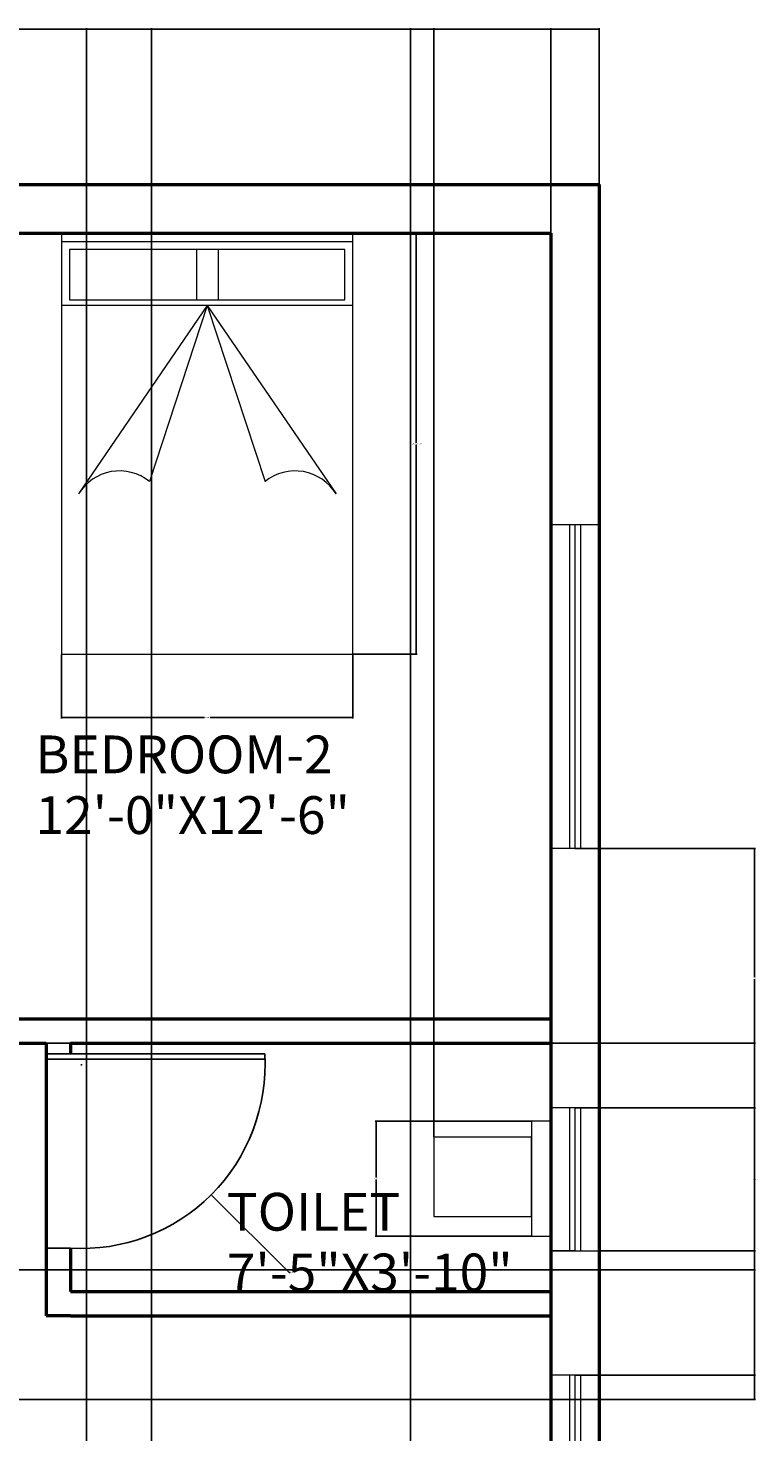
# Model space of a CAD drawing. Units: inches. Extents: x 2750 to 3097, y 1429 to 2028.
# Tile 4 of 4: x 2962 to 3097, y 1768 to 2028. Entities that reach past the tile are written whole.
import ezdxf

# ---------------------------------------------------------------- set-up
doc = ezdxf.new("R2010")
doc.units = ezdxf.units.IN
for name, color, linetype, lineweight in [('A-ANNO-DIMS', 2, 'Continuous', 18), ('A-AREA-IDEN', 7, 'Continuous', 25), ('A-DOOR', 3, 'Continuous', 25), ('A-FLOR-FIXT', 9, 'Continuous', 18), ('A-FURN', 8, 'Continuous', 18), ('A-GLAZ', 4, 'Continuous', 18), ('A-WALL', 7, 'Continuous', 50)]:
    doc.layers.add(name, color=color, linetype=linetype, lineweight=lineweight)
doc.styles.get("Standard").update_dxf_attribs({"font": 'arial.ttf'})
doc.dimstyles.get("Standard").update_dxf_attribs({"dimtxt": 0.18, "dimasz": 0.18, "dimexe": 0.18, "dimexo": 0.0625, "dimgap": 0.09, "dimtad": 0, "dimtih": 1, "dimtoh": 1, "dimdec": 4, "dimzin": 0, "dimdsep": 46, "dimtxsty": 'Standard', "dimcen": 0.09, "dimadec": 0, "dimazin": 0, "dimtfac": 1, "dimtdec": 4, "dimtofl": 0, "dimtmove": 0, "dimatfit": 3, "dimfxl": 1, "dimtolj": 1, "dimtzin": 0, "dimarcsym": 0})

# ---------------------------------------------------------------- blocks, each defined once
blk = doc.blocks.new('BED-DOUBLE-54X78')
for p, q in [((0, 78), (0, 0)), ((54, 78), (0, 78)), ((54, 0), (54, 78)), ((27, 13.39), (3.13, 48.31)), ((27, 13.39), (50.87, 48.31)), ((27, 13.39), (16.28, 45.98)), ((27, 13.39), (37.72, 45.98)), ((0, 13.39), (54, 13.39)), ((24.99, 3.04), (24.99, 12.35)), ((28.99, 3.04), (28.99, 12.35)), ((0, 1.59), (54, 1.59)), ((0, 0), (54, 0))]:
    blk.add_line(p, q)
blk.add_lwpolyline([(1.48, 3.04), (52.5, 3.04), (52.5, 12.35), (1.48, 12.35)], close=True)
for centre, start, end in [((10.73, 52.93), 211.2898, 308.6091), ((43.27, 52.93), 231.3909, 328.7102)]:
    blk.add_arc(centre, 8.89, start, end)
blk = doc.blocks.new('WIN-60IN')
for p, q in [((9, 60), (0, 60)), ((3.5, 60), (3.5, 0)), ((4.5, 60), (4.5, 0)), ((5.5, 60), (5.5, 0)), ((9, 0), (0, 0))]:
    blk.add_line(p, q)
blk = doc.blocks.new('*D9')
at = {"layer": 'A-ANNO-DIMS', "color": 0, "lineweight": -2, "transparency": 16777216}
for p, q in [((3021.93, 1989.59), (3033.75, 1989.59)), ((3033.57, 1989.41), (3033.57, 1950.78)), ((3033.57, 1911.77), (3033.57, 1950.41)), ((3021.93, 1911.59), (3033.75, 1911.59))]:
    blk.add_line(p, q, dxfattribs=at)
at = {"layer": 'A-ANNO-DIMS', "color": 0, "transparency": 16777216}
for points in [[(3033.54, 1989.41), (3033.6, 1989.41), (3033.57, 1989.59)], [(3033.54, 1911.77), (3033.6, 1911.77), (3033.57, 1911.59)]]:
    blk.add_solid(points, dxfattribs=at)
at = {"layer": 'Defpoints', "color": 0, "transparency": 16777216}
for p in [(3021.87, 1989.59), (3021.87, 1911.59), (3033.57, 1911.59)]:
    blk.add_point(p, dxfattribs=at)
at = {"layer": 'A-ANNO-DIMS', "color": 0, "transparency": 16777216, "insert": (3033.57, 1950.59), "char_height": 0.18, "attachment_point": 5}
blk.add_mtext('\\A1;DOUBLE BED 78 TYP.', dxfattribs=at)
blk = doc.blocks.new('*D10')
at = {"layer": 'A-ANNO-DIMS', "color": 0, "lineweight": -2, "transparency": 16777216}
for p, q in [((2967.87, 1911.53), (2967.87, 1899.71)), ((3021.87, 1911.53), (3021.87, 1899.71)), ((2968.05, 1899.89), (2994.34, 1899.89)), ((3021.69, 1899.89), (2995.4, 1899.89))]:
    blk.add_line(p, q, dxfattribs=at)
at = {"layer": 'A-ANNO-DIMS', "color": 0, "transparency": 16777216}
for points in [[(2968.05, 1899.92), (2968.05, 1899.86), (2967.87, 1899.89)], [(3021.69, 1899.92), (3021.69, 1899.86), (3021.87, 1899.89)]]:
    blk.add_solid(points, dxfattribs=at)
at = {"layer": 'Defpoints', "color": 0, "transparency": 16777216}
for p in [(2967.87, 1911.59), (3021.87, 1911.59), (2967.87, 1899.89)]:
    blk.add_point(p, dxfattribs=at)
at = {"layer": 'A-ANNO-DIMS', "color": 0, "transparency": 16777216, "insert": (2994.87, 1899.89), "char_height": 0.18, "attachment_point": 5}
blk.add_mtext('\\A1;54 TYP.', dxfattribs=at)
blk = doc.blocks.new('*D13')
at = {"layer": 'A-ANNO-DIMS', "color": 0, "lineweight": -2, "transparency": 16777216}
for p, q in [((2779.52, 1998.66), (2779.52, 2027.57)), ((2779.7, 2027.39), (2923.23, 2027.39)), ((3067.34, 2027.39), (2923.81, 2027.39)), ((3067.52, 1998.66), (3067.52, 2027.57))]:
    blk.add_line(p, q, dxfattribs=at)
at = {"layer": 'A-ANNO-DIMS', "color": 0, "transparency": 16777216}
for points in [[(2779.7, 2027.42), (2779.7, 2027.36), (2779.52, 2027.39)], [(3067.34, 2027.42), (3067.34, 2027.36), (3067.52, 2027.39)]]:
    blk.add_solid(points, dxfattribs=at)
at = {"layer": 'Defpoints', "color": 0, "transparency": 16777216}
for p in [(3067.52, 2027.39), (2779.52, 1998.59), (3067.52, 1998.59)]:
    blk.add_point(p, dxfattribs=at)
at = {"layer": 'A-ANNO-DIMS', "color": 0, "transparency": 16777216, "insert": (2923.52, 2027.39), "char_height": 0.18, "attachment_point": 5}
blk.add_mtext('\\A1;288', dxfattribs=at)
blk = doc.blocks.new('*D27')
at = {"layer": 'A-ANNO-DIMS', "color": 0, "lineweight": -2, "transparency": 16777216}
for p, q in [((3067.58, 1801.09), (3096.5, 1801.09)), ((3096.32, 1800.91), (3096.32, 1789.77)), ((3096.32, 1778.27), (3096.32, 1789.41)), ((3067.58, 1778.09), (3096.5, 1778.09))]:
    blk.add_line(p, q, dxfattribs=at)
at = {"layer": 'A-ANNO-DIMS', "color": 0, "transparency": 16777216}
for points in [[(3096.29, 1800.91), (3096.35, 1800.91), (3096.32, 1801.09)], [(3096.29, 1778.27), (3096.35, 1778.27), (3096.32, 1778.09)]]:
    blk.add_solid(points, dxfattribs=at)
at = {"layer": 'Defpoints', "color": 0, "transparency": 16777216}
for p in [(3067.52, 1801.09), (3096.32, 1801.09), (3067.52, 1778.09)]:
    blk.add_point(p, dxfattribs=at)
at = {"layer": 'A-ANNO-DIMS', "color": 0, "transparency": 16777216, "insert": (3096.32, 1789.59), "char_height": 0.18, "attachment_point": 5}
blk.add_mtext('\\A1;23', dxfattribs=at)
blk = doc.blocks.new('*D28')
at = {"layer": 'A-ANNO-DIMS', "color": 0, "lineweight": -2, "transparency": 16777216}
for p, q in [((3067.58, 1827.59), (3096.5, 1827.59)), ((3096.32, 1827.41), (3096.32, 1814.52)), ((3096.32, 1801.27), (3096.32, 1814.16)), ((3067.58, 1801.09), (3096.5, 1801.09))]:
    blk.add_line(p, q, dxfattribs=at)
at = {"layer": 'A-ANNO-DIMS', "color": 0, "transparency": 16777216}
for points in [[(3096.29, 1827.41), (3096.35, 1827.41), (3096.32, 1827.59)], [(3096.29, 1801.27), (3096.35, 1801.27), (3096.32, 1801.09)]]:
    blk.add_solid(points, dxfattribs=at)
at = {"layer": 'Defpoints', "color": 0, "transparency": 16777216}
for p in [(3067.52, 1827.59), (3096.32, 1827.59), (3067.52, 1801.09)]:
    blk.add_point(p, dxfattribs=at)
at = {"layer": 'A-ANNO-DIMS', "color": 0, "transparency": 16777216, "insert": (3096.32, 1814.34), "char_height": 0.18, "attachment_point": 5}
blk.add_mtext('\\A1;26.5', dxfattribs=at)
blk = doc.blocks.new('*D29')
at = {"layer": 'A-ANNO-DIMS', "color": 0, "lineweight": -2, "transparency": 16777216}
for p, q in [((3067.58, 1875.59), (3096.5, 1875.59)), ((3096.32, 1875.41), (3096.32, 1851.77)), ((3096.32, 1827.77), (3096.32, 1851.41)), ((3067.58, 1827.59), (3096.5, 1827.59))]:
    blk.add_line(p, q, dxfattribs=at)
at = {"layer": 'A-ANNO-DIMS', "color": 0, "transparency": 16777216}
for points in [[(3096.29, 1875.41), (3096.35, 1875.41), (3096.32, 1875.59)], [(3096.29, 1827.77), (3096.35, 1827.77), (3096.32, 1827.59)]]:
    blk.add_solid(points, dxfattribs=at)
at = {"layer": 'Defpoints', "color": 0, "transparency": 16777216}
for p in [(3067.52, 1875.59), (3096.32, 1875.59), (3067.52, 1827.59)]:
    blk.add_point(p, dxfattribs=at)
at = {"layer": 'A-ANNO-DIMS', "color": 0, "transparency": 16777216, "insert": (3096.32, 1851.59), "char_height": 0.18, "attachment_point": 5}
blk.add_mtext('\\A1;48', dxfattribs=at)
blk = doc.blocks.new('*D36')
at = {"layer": 'A-ANNO-DIMS', "color": 0, "lineweight": -2, "transparency": 16777216}
for p, q in [((3036.87, 1822.2), (3036.87, 2027.57)), ((3037.05, 2027.39), (3047.23, 2027.39)), ((3058.34, 2027.39), (3048.16, 2027.39)), ((3058.52, 1825.17), (3058.52, 2027.57))]:
    blk.add_line(p, q, dxfattribs=at)
at = {"layer": 'A-ANNO-DIMS', "color": 0, "transparency": 16777216}
for points in [[(3037.05, 2027.42), (3037.05, 2027.36), (3036.87, 2027.39)], [(3058.34, 2027.42), (3058.34, 2027.36), (3058.52, 2027.39)]]:
    blk.add_solid(points, dxfattribs=at)
at = {"layer": 'Defpoints', "color": 0, "transparency": 16777216}
for p in [(3058.52, 2027.39), (3058.52, 1825.11), (3036.87, 1822.14)]:
    blk.add_point(p, dxfattribs=at)
at = {"layer": 'A-ANNO-DIMS', "color": 0, "transparency": 16777216, "insert": (3047.69, 2027.39), "char_height": 0.18, "attachment_point": 5}
blk.add_mtext('\\A1;21.652', dxfattribs=at)
blk = doc.blocks.new('*D37')
at = {"layer": 'A-ANNO-DIMS', "color": 0, "lineweight": -2, "transparency": 16777216}
for p, q in [((3054.91, 1825.11), (3026, 1825.11)), ((3026.18, 1824.93), (3026.18, 1814.66)), ((3026.18, 1804.02), (3026.18, 1814.29)), ((3054.91, 1803.84), (3026, 1803.84))]:
    blk.add_line(p, q, dxfattribs=at)
at = {"layer": 'A-ANNO-DIMS', "color": 0, "transparency": 16777216}
for points in [[(3026.15, 1824.93), (3026.21, 1824.93), (3026.18, 1825.11)], [(3026.15, 1804.02), (3026.21, 1804.02), (3026.18, 1803.84)]]:
    blk.add_solid(points, dxfattribs=at)
at = {"layer": 'Defpoints', "color": 0, "transparency": 16777216}
for p in [(3026.18, 1825.11), (3054.98, 1825.11), (3054.98, 1803.84)]:
    blk.add_point(p, dxfattribs=at)
at = {"layer": 'A-ANNO-DIMS', "color": 0, "transparency": 16777216, "insert": (3026.18, 1814.47), "char_height": 0.18, "attachment_point": 5}
blk.add_mtext('\\A1;21.266', dxfattribs=at)
blk = doc.blocks.new('*D40')
at = {"layer": 'A-ANNO-DIMS', "color": 0, "lineweight": -2, "transparency": 16777216}
for p, q in [((2860.58, 1797.59), (3096.5, 1797.59)), ((3096.32, 1797.41), (3096.32, 1785.77)), ((3096.32, 1773.77), (3096.32, 1785.41)), ((2860.58, 1773.59), (3096.5, 1773.59))]:
    blk.add_line(p, q, dxfattribs=at)
at = {"layer": 'A-ANNO-DIMS', "color": 0, "transparency": 16777216}
for points in [[(3096.29, 1797.41), (3096.35, 1797.41), (3096.32, 1797.59)], [(3096.29, 1773.77), (3096.35, 1773.77), (3096.32, 1773.59)]]:
    blk.add_solid(points, dxfattribs=at)
at = {"layer": 'Defpoints', "color": 0, "transparency": 16777216}
for p in [(2860.52, 1797.59), (3096.32, 1797.59), (2860.52, 1773.59)]:
    blk.add_point(p, dxfattribs=at)
at = {"layer": 'A-ANNO-DIMS', "color": 0, "transparency": 16777216, "insert": (3096.32, 1785.59), "char_height": 0.18, "attachment_point": 5}
blk.add_mtext('\\A1;24', dxfattribs=at)
blk = doc.blocks.new('*D41')
at = {"layer": 'A-ANNO-DIMS', "color": 0, "lineweight": -2, "transparency": 16777216}
for p, q in [((2865.08, 1839.59), (3096.5, 1839.59)), ((3096.32, 1839.41), (3096.32, 1818.77)), ((3096.32, 1797.77), (3096.32, 1818.41)), ((2865.08, 1797.59), (3096.5, 1797.59))]:
    blk.add_line(p, q, dxfattribs=at)
at = {"layer": 'A-ANNO-DIMS', "color": 0, "transparency": 16777216}
for points in [[(3096.29, 1839.41), (3096.35, 1839.41), (3096.32, 1839.59)], [(3096.29, 1797.77), (3096.35, 1797.77), (3096.32, 1797.59)]]:
    blk.add_solid(points, dxfattribs=at)
at = {"layer": 'Defpoints', "color": 0, "transparency": 16777216}
for p in [(2865.02, 1839.59), (3096.32, 1839.59), (2865.02, 1797.59)]:
    blk.add_point(p, dxfattribs=at)
at = {"layer": 'A-ANNO-DIMS', "color": 0, "transparency": 16777216, "insert": (3096.32, 1818.59), "char_height": 0.18, "attachment_point": 5}
blk.add_mtext('\\A1;42', dxfattribs=at)
blk = doc.blocks.new('*D51')
at = {"layer": 'A-ANNO-DIMS', "color": 0, "lineweight": -2, "transparency": 16777216}
for p, q in [((2972.52, 1605.66), (2972.52, 2027.57)), ((2972.7, 2027.39), (2978.31, 2027.39)), ((2984.34, 2027.39), (2978.73, 2027.39)), ((2984.52, 1605.66), (2984.52, 2027.57))]:
    blk.add_line(p, q, dxfattribs=at)
at = {"layer": 'A-ANNO-DIMS', "color": 0, "transparency": 16777216}
for points in [[(2972.7, 2027.42), (2972.7, 2027.36), (2972.52, 2027.39)], [(2984.34, 2027.42), (2984.34, 2027.36), (2984.52, 2027.39)]]:
    blk.add_solid(points, dxfattribs=at)
at = {"layer": 'Defpoints', "color": 0, "transparency": 16777216}
for p in [(2984.52, 2027.39), (2972.52, 1605.59), (2984.52, 1605.59)]:
    blk.add_point(p, dxfattribs=at)
at = {"layer": 'A-ANNO-DIMS', "color": 0, "transparency": 16777216, "insert": (2978.52, 2027.39), "char_height": 0.18, "attachment_point": 5}
blk.add_mtext('\\A1;12', dxfattribs=at)
blk = doc.blocks.new('*D52')
at = {"layer": 'A-ANNO-DIMS', "color": 0, "lineweight": -2, "transparency": 16777216}
for p, q in [((2908.52, 1605.66), (2908.52, 2027.57)), ((2908.7, 2027.39), (2940.3, 2027.39)), ((2972.34, 2027.39), (2940.74, 2027.39)), ((2972.52, 1605.66), (2972.52, 2027.57))]:
    blk.add_line(p, q, dxfattribs=at)
at = {"layer": 'A-ANNO-DIMS', "color": 0, "transparency": 16777216}
for points in [[(2908.7, 2027.42), (2908.7, 2027.36), (2908.52, 2027.39)], [(2972.34, 2027.42), (2972.34, 2027.36), (2972.52, 2027.39)]]:
    blk.add_solid(points, dxfattribs=at)
at = {"layer": 'Defpoints', "color": 0, "transparency": 16777216}
for p in [(2972.52, 2027.39), (2908.52, 1605.59), (2972.52, 1605.59)]:
    blk.add_point(p, dxfattribs=at)
at = {"layer": 'A-ANNO-DIMS', "color": 0, "transparency": 16777216, "insert": (2940.52, 2027.39), "char_height": 0.18, "attachment_point": 5}
blk.add_mtext('\\A1;64', dxfattribs=at)
blk = doc.blocks.new('*D53')
at = {"layer": 'A-ANNO-DIMS', "color": 0, "lineweight": -2, "transparency": 16777216}
for p, q in [((3032.52, 1605.66), (3032.52, 2027.57)), ((3032.7, 2027.39), (3045.3, 2027.39)), ((3058.34, 2027.39), (3045.74, 2027.39)), ((3058.52, 1605.66), (3058.52, 2027.57))]:
    blk.add_line(p, q, dxfattribs=at)
at = {"layer": 'A-ANNO-DIMS', "color": 0, "transparency": 16777216}
for points in [[(3032.7, 2027.42), (3032.7, 2027.36), (3032.52, 2027.39)], [(3058.34, 2027.42), (3058.34, 2027.36), (3058.52, 2027.39)]]:
    blk.add_solid(points, dxfattribs=at)
at = {"layer": 'Defpoints', "color": 0, "transparency": 16777216}
for p in [(3058.52, 2027.39), (3032.52, 1605.59), (3058.52, 1605.59)]:
    blk.add_point(p, dxfattribs=at)
at = {"layer": 'A-ANNO-DIMS', "color": 0, "transparency": 16777216, "insert": (3045.52, 2027.39), "char_height": 0.18, "attachment_point": 5}
blk.add_mtext('\\A1;26', dxfattribs=at)
blk = doc.blocks.new('*D65')
at = {"layer": 'A-ANNO-DIMS', "color": 0, "lineweight": -2, "transparency": 16777216}
for p, q in [((2971.46, 1835.56), (2971.64, 1835.56)), ((2971.55, 1835.47), (2971.55, 1835.65)), ((3010.05, 1797.06), (2995.74, 1811.37)), ((3010.23, 1797.06), (3010.05, 1797.06))]:
    blk.add_line(p, q, dxfattribs=at)
at = {"layer": 'A-ANNO-DIMS', "color": 0, "transparency": 16777216}
blk.add_solid([(2995.76, 1811.39), (2995.72, 1811.35), (2995.61, 1811.5)], dxfattribs=at)
at = {"layer": 'Defpoints', "color": 0, "transparency": 16777216}
for p in [(2971.55, 1835.56), (2995.61, 1811.5)]:
    blk.add_point(p, dxfattribs=at)
at = {"layer": 'A-ANNO-DIMS', "color": 0, "transparency": 16777216, "insert": (3010.71, 1797.06), "char_height": 0.18, "attachment_point": 5}
blk.add_mtext('\\A1;R34.03', dxfattribs=at)

msp = doc.modelspace()

# ---------------------------------------------------------------- linework, layer by layer
at = {"layer": 'A-DOOR'}
for p, q in [((2969.5201, 1837.5925), (2965.0201, 1837.5925)), ((2969.5201, 1836.5925), (2965.0201, 1836.5925)), ((2969.5201, 1837.5925), (3005.5201, 1837.5925)), ((2969.5201, 1836.5925), (3005.5201, 1836.5925)), ((2969.5201, 1801.5925), (2965.0201, 1801.5925))]:
    msp.add_line(p, q, dxfattribs=at)
msp.add_arc((2971.5518, 1835.5609), 34.029, 266.577182, 3.422818, dxfattribs=at)
at = {"layer": 'A-FLOR-FIXT'}
for p, q in [((3058.5201, 1825.1067), (3054.9767, 1825.1067)), ((3054.9767, 1825.1067), (3054.9767, 1803.8407)), ((3054.9767, 1803.8407), (3058.5201, 1803.8407))]:
    msp.add_line(p, q, dxfattribs=at)
msp.add_lwpolyline([(3054.9767, 1822.1388), (3036.8677, 1822.1388), (3036.8677, 1807.4726), (3054.9767, 1807.4726)], close=True, dxfattribs=at)
at = {"layer": 'A-GLAZ'}
for p, q in [((3063.0201, 1875.5925), (3067.5201, 1875.5925)), ((3067.5201, 1827.5925), (3058.5201, 1827.5925)), ((3062.0201, 1827.5925), (3062.0201, 1801.0925)), ((3063.0201, 1827.5925), (3067.5201, 1827.5925)), ((3063.0201, 1827.5925), (3063.0201, 1801.0925)), ((3064.0201, 1827.5925), (3064.0201, 1801.0925)), ((3063.0201, 1801.0925), (3058.5201, 1801.0925)), ((3058.5201, 1801.0925), (3067.5201, 1801.0925)), ((3067.5201, 1778.0925), (3058.5201, 1778.0925)), ((3062.0172, 1778.0925), (3062.0172, 1742.0925)), ((3063.0172, 1778.0925), (3067.5201, 1778.0925)), ((3063.0172, 1778.0925), (3063.0172, 1742.0925)), ((3064.0172, 1778.0925), (3064.0172, 1742.0925))]:
    msp.add_line(p, q, dxfattribs=at)
at = {"layer": 'A-WALL'}
for p, q in [((2779.5201, 1998.5925), (3067.5201, 1998.5925)), ((3067.5201, 1998.5925), (3067.5201, 1494.5925)), ((2788.5201, 1989.5925), (3058.5201, 1989.5925)), ((3058.5201, 1989.5925), (3058.5201, 1503.5925)), ((2953.5201, 1844.0925), (3058.5201, 1844.0925)), ((2788.5201, 1839.5925), (2965.0201, 1839.5925)), ((2965.0201, 1839.5925), (2965.0201, 1793.5925)), ((2969.5201, 1839.5925), (2969.5201, 1837.5925)), ((2969.5201, 1839.5925), (2969.5201, 1837.5925)), ((2969.5201, 1839.5925), (3058.5201, 1839.5925)), ((2969.5201, 1801.5925), (2969.5201, 1793.5925)), ((2965.0201, 1793.5925), (2965.0201, 1789.0925)), ((2969.5201, 1793.5925), (3058.5201, 1793.5925)), ((2969.5201, 1789.0925), (2965.0201, 1789.0925)), ((2969.5201, 1789.0925), (3058.5201, 1789.0925))]:
    msp.add_line(p, q, dxfattribs=at)

# ---------------------------------------------------------------- block references
at = {"layer": 'A-FURN', "rotation": 180}
msp.add_blockref('BED-DOUBLE-54X78', (3021.8714, 1989.5927), dxfattribs=at)
at = {"layer": 'A-GLAZ'}
msp.add_blockref('WIN-60IN', (3058.52, 1875.593), dxfattribs=at)

# ---------------------------------------------------------------- texts
at = {"layer": 'A-AREA-IDEN'}
for s, p in [('BEDROOM-2', (2963.0451, 1889.5498)), ('12\'-0"X12\'-6"', (2963.0451, 1878.305)), ('TOILET', (2998.5089, 1804.8374)), ('7\'-5"X3\'-10"', (2998.5089, 1793.5925))]:
    msp.add_text(s, height=7, dxfattribs=at).set_placement(p)

# ---------------------------------------------------------------- dimensions: what is measured, and where the dimension line sits
at = {"layer": 'A-ANNO-DIMS'}
for base, p1, p2, override, picture, middle in [((3067.5201, 2027.3925), (2779.5201, 1998.5925), (3067.5201, 1998.5925), {"dimdec": 0, "dimlfac": 1, "dimrnd": 0, "dimzin": 0, "dimdsep": 46, "dimlunit": 2}, '*D13', (2923.5201, 2027.3925)), ((2972.5201, 2027.3925), (2908.5201, 1605.5925), (2972.5201, 1605.5925), {"dimdec": 0, "dimlfac": 1, "dimrnd": 0, "dimzin": 0, "dimdsep": 46, "dimlunit": 2}, '*D52', (2940.5201, 2027.3925)), ((2984.5201, 2027.3925), (2972.5201, 1605.5925), (2984.5201, 1605.5925), {"dimdec": 0, "dimlfac": 1, "dimrnd": 0, "dimzin": 0, "dimdsep": 46, "dimlunit": 2}, '*D51', (2978.5201, 2027.3925)), ((3058.5201, 2027.3925), (3032.5201, 1605.5925), (3058.5201, 1605.5925), {"dimdec": 0, "dimlfac": 1, "dimrnd": 0, "dimzin": 0, "dimdsep": 46, "dimlunit": 2}, '*D53', (3045.5201, 2027.3925)), ((3058.5201, 2027.3925), (3036.8677, 1822.1388), (3058.5201, 1825.1067), {"dimdec": 3, "dimlfac": 1, "dimrnd": 0, "dimzin": 0, "dimdsep": 46, "dimlunit": 2}, '*D36', (3047.6939, 2027.3925))]:
    dim = msp.add_linear_dim(base=base, p1=p1, p2=p2, dimstyle='Standard', override=override, dxfattribs=at)
    dim.commit()
    dim.dimension.update_dxf_attribs({"geometry": picture, "text_midpoint": middle})
for base, p1, p2, angle, text, picture, middle in [((3033.5718, 1911.5925), (3021.8718, 1989.5925), (3021.8718, 1911.5925), 270, 'DOUBLE BED <> TYP.', '*D9', (3033.5718, 1950.5925)), ((2967.8718, 1899.8925), (3021.8718, 1911.5925), (2967.8718, 1911.5925), 180, '<> TYP.', '*D10', (2994.8718, 1899.8925))]:
    dim = msp.add_linear_dim(base=base, p1=p1, p2=p2, angle=angle, text=text, dimstyle='Standard', override={"dimdec": 0, "dimlfac": 1, "dimrnd": 0, "dimzin": 0, "dimdsep": 46, "dimlunit": 2}, dxfattribs=at)
    dim.commit()
    dim.dimension.update_dxf_attribs({"geometry": picture, "text_midpoint": middle})
for base, p1, p2, override, picture, middle in [((3096.3201, 1875.5925), (3067.5201, 1827.5925), (3067.5201, 1875.5925), {"dimdec": 0, "dimlfac": 1, "dimrnd": 0, "dimzin": 0, "dimdsep": 46, "dimlunit": 2}, '*D29', (3096.3201, 1851.5925)), ((3096.3201, 1839.5925), (2865.0201, 1797.5925), (2865.0201, 1839.5925), {"dimdec": 0, "dimlfac": 1, "dimrnd": 0, "dimzin": 0, "dimdsep": 46, "dimlunit": 2}, '*D41', (3096.3201, 1818.5925)), ((3096.3201, 1827.5925), (3067.5201, 1801.0925), (3067.5201, 1827.5925), {"dimdec": 1, "dimlfac": 1, "dimrnd": 0, "dimzin": 0, "dimdsep": 46, "dimlunit": 2}, '*D28', (3096.3201, 1814.3425)), ((3026.1767, 1825.1067), (3054.9767, 1803.8407), (3054.9767, 1825.1067), {"dimdec": 3, "dimlfac": 1, "dimrnd": 0, "dimzin": 0, "dimdsep": 46, "dimlunit": 2}, '*D37', (3026.1767, 1814.4737)), ((3096.3201, 1801.0925), (3067.5201, 1778.0925), (3067.5201, 1801.0925), {"dimdec": 0, "dimlfac": 1, "dimrnd": 0, "dimzin": 0, "dimdsep": 46, "dimlunit": 2}, '*D27', (3096.3201, 1789.5925)), ((3096.3201, 1797.5925), (2860.5201, 1773.5925), (2860.5201, 1797.5925), {"dimdec": 0, "dimlfac": 1, "dimrnd": 0, "dimzin": 0, "dimdsep": 46, "dimlunit": 2}, '*D40', (3096.3201, 1785.5925))]:
    dim = msp.add_linear_dim(base=base, p1=p1, p2=p2, angle=90, dimstyle='Standard', override=override, dxfattribs=at)
    dim.commit()
    dim.dimension.update_dxf_attribs({"geometry": picture, "text_midpoint": middle})
dim = msp.add_radius_dim(center=(2971.5518, 1835.5609), mpoint=(2995.6141, 1811.4989), dimstyle='Standard', override={"dimdec": 2, "dimlfac": 1, "dimrnd": 0, "dimzin": 0, "dimdsep": 46, "dimlunit": 2}, dxfattribs=at)
dim.commit()
dim.dimension.update_dxf_attribs({"geometry": '*D65', "text_midpoint": (3010.7114, 1797.0617), "dimtype": 164})

doc.saveas('drawing.dxf')
